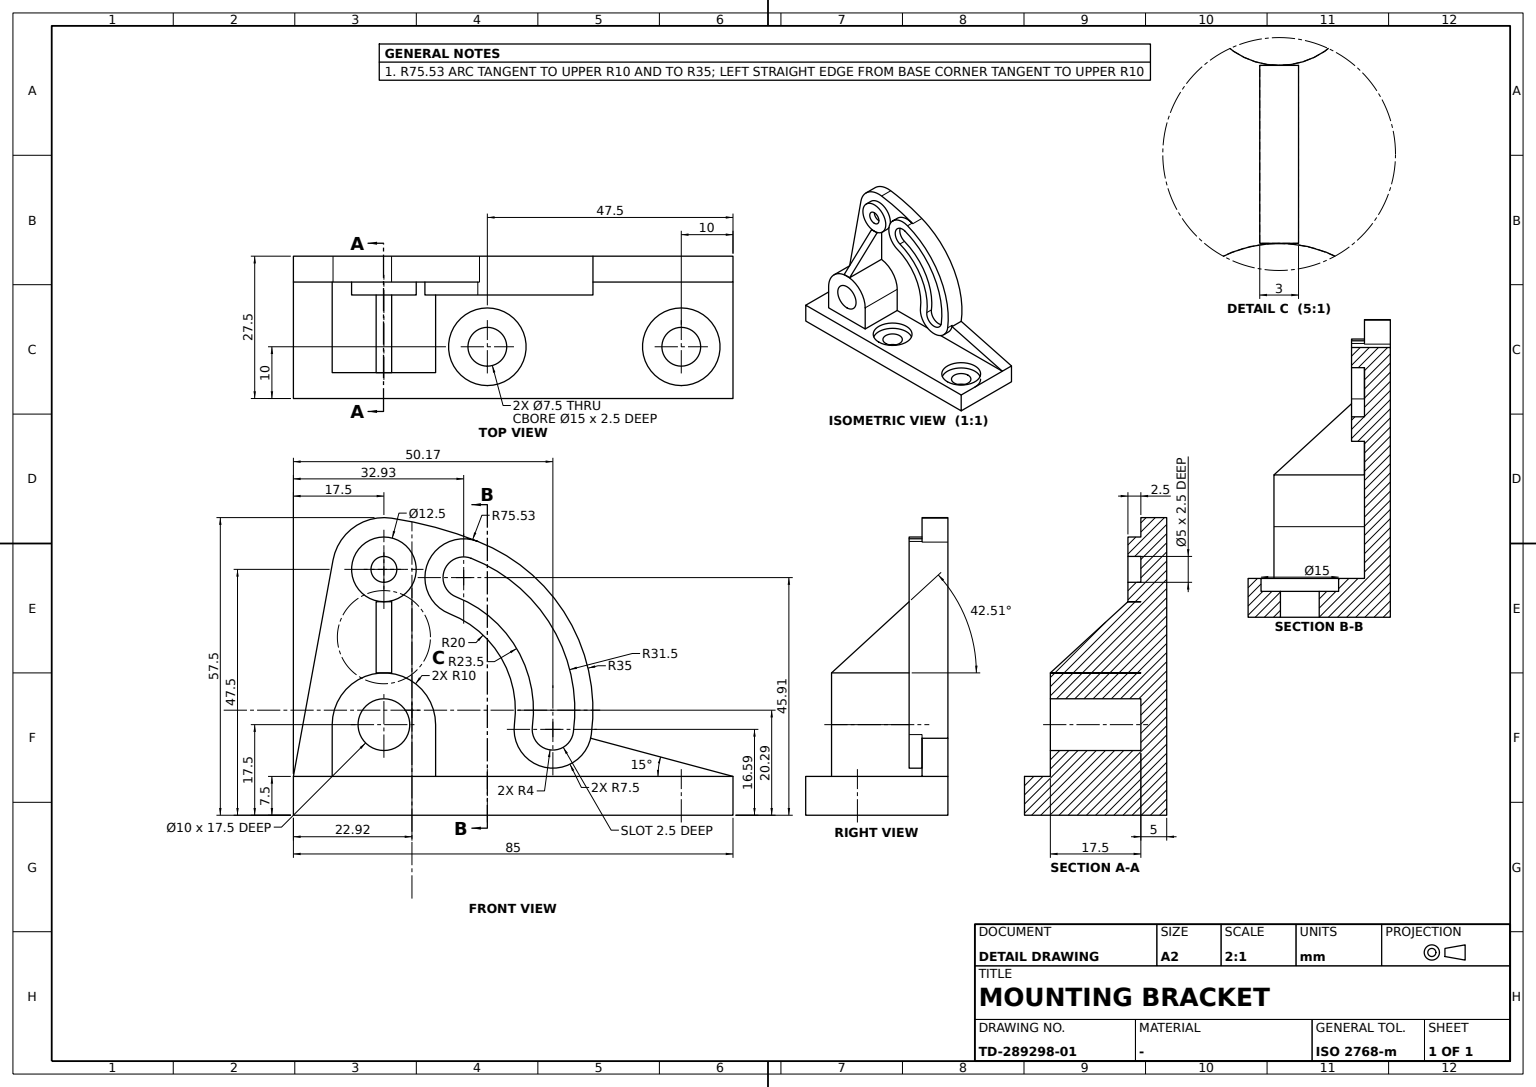
CATIA V5 part; units mm, degrees
sketch "Sketch1" plane through (0, 0, 0) normal (0, 0, 1) x (1, 0, 0)
  line L0 (13.75, 42.5) -> (13.75, -42.5)
  line L1 (13.75, -42.5) -> (-13.75, -42.5)
  line L2 (-13.75, -42.5) -> (-13.75, 42.5)
  line L3 (-13.75, 42.5) -> (13.75, 42.5)
  dimension "length L0" = 85
  dimension "length L1" = 27.5
  constraint vertical L0 y-axis
  constraint vertical L2 y-axis
  constraint horizontal L1 x-axis
  constraint horizontal L3 x-axis
  constraint equidistance L0 L2 origin
  constraint equidistance L1 L3 origin
extrude "Pad1" add sketch "Sketch1" along normal blind 7.5
sketch "Sketch2" plane through (-13.75, 0, 0) normal (-1, 0, 0) x (0, -1, 0)
  arc A0 (34.8361, 49.3033) -> (23.5195, 57.3898) centre (25, 47.5) ccw
  point P0 (25, 47.5)
  line L0 (-42.5, 7.5) -> (42.5, 7.5) construction
  line L1 (42.5, 0) -> (42.5, 7.5) construction
  line L2 (34.8361, 49.3033) -> (42.5, 7.5)
  point P1 (42.5, 7.5)
  point P2 (42.5, 7.5)
  point P3 (25, 17.5)
  line L3 (-42.5, 7.5) -> (42.5, 7.5) construction
  line L4 (42.5, 0) -> (42.5, 7.5) construction
  line L5 (-42.5, 7.5) -> (-15, 14.8686)
  point P4 (-42.5, 7.5)
  point P5 (-42.5, 7.5)
  line L6 (-42.5, 7.5) -> (42.5, 7.5) construction
  line L7 (-42.5, 7.5) -> (42.5, 7.5)
  point P6 (9.75, 46.2)
  arc A1 (-15, 14.8686) -> (6.5158, 52.7659) centre (19.5769, 20.2943) cw
  point P7 (-15, 14.8686)
  point P8 (6.5158, 52.7659)
  arc A2 (6.5158, 52.7659) -> (23.5195, 57.3898) centre (34.7021, -17.309) cw
  point P9 (6.5158, 52.7659)
  arc A3 (13.3911, 47.8559) -> (-6.4867, 9.4478) centre (25, 17.5) ccw construction
  point P10 (-15, 14.8686)
  dimension "distance P0 L0" = 40
  dimension "radius A0" = 10
  dimension "distance P0 L1" = 17.5
  dimension "distance P3 L3" = 10
  dimension "distance P3 L4" = 17.5
  dimension "angle L6 L5" = 15
  dimension "distance P6 P0 x axis" = 15.25
  dimension "radius A1" = 35
  dimension "radius A2" = 75.5312
  dimension "distance P7 P0 x axis" = 40
  constraint coincidence P2 P1
  constraint coincidence P5 P4
  constraint coincidence P7 P10
  constraint coincidence P8 P9
  constraint tangency L2 A0
  constraint tangency A0 A2
  constraint tangency A1 A2
  constraint horizontal L7 x-axis
extrude "Pad2" add sketch "Sketch2" against normal blind 5
sketch "Sketch3" plane through (-8.75, 0, 0) normal (1, 0, 0) x (0, 1, 0)
  point P0 (-6.92, 52.9252)
  point P1 (-13.2128, 47.5656)
  point P2 (6.665, 9.1574)
  point P3 (14.9168, 14.6483)
  point P4 (7.6724, 16.5895)
  point P5 (-9.5717, 45.9096)
  point P6 (-19.5769, 20.2943)
  arc A0 (-13.2128, 47.5656) -> (6.665, 9.1574) centre (-24.8217, 17.2096) cw construction
  point P7 (-19.5769, 20.2943)
  arc A1 (-11.027, 42.1837) -> (-8.1164, 49.6355) centre (-9.5717, 45.9096) cw
  arc A2 (15.104, 15.579) -> (0.2408, 17.5999) centre (7.6724, 16.5895) cw
  arc A3 (15.104, 15.579) -> (-6.843, 52.8956) centre (-19.5769, 20.2943) ccw
  arc A4 (-12.3004, 38.9236) -> (-6.843, 52.8956) centre (-9.5717, 45.9096) cw
  arc A5 (0.2408, 17.5999) -> (-12.3004, 38.9236) centre (-19.5769, 20.2943) ccw
  arc A6 (-11.027, 42.1837) -> (3.7089, 17.1283) centre (-19.5769, 20.2943) cw
  arc A7 (11.6359, 16.0506) -> (3.7089, 17.1283) centre (7.6724, 16.5895) cw
  arc A8 (-8.1164, 49.6355) -> (11.6359, 16.0506) centre (-19.5769, 20.2943) cw
  arc A9 (15, 14.8686) -> (-6.5158, 52.7659) centre (-19.5769, 20.2943) ccw construction
  dimension "radius A2" = 7.5
  dimension "radius A7" = 4
  dimension "radius A0" = 32.5
  constraint coincidence P0 A4
  constraint coincidence P1 A1
  constraint coincidence P2 A2
  constraint coincidence P3 A2
  constraint coincidence P4 A0
  constraint coincidence P5 A0
  constraint coincidence P6 P7
  constraint coincidence A3 A9
  constraint concentricity P6 A5
  constraint concentricity P6 A6
  constraint concentricity P6 A8
  constraint tangency A1 A6
  constraint tangency A1 A8
  constraint tangency A2 A3
  constraint tangency A2 A5
  constraint tangency A3 A4
  constraint tangency A4 A5
  constraint tangency A6 A7
  constraint tangency A7 A8
extrude "Pad3" add sketch "Sketch3" along normal blind 2.5
sketch "Sketch4" plane through (-8.75, 0, 0) normal (1, 0, 0) x (0, 1, 0)
  arc A0 (-15, 17.5) -> (-35, 17.5) centre (-25, 17.5) ccw
  point P0 (-25, 17.5)
  line L0 (-42.5, 0) -> (-42.5, 7.5) construction
  line L1 (-42.5, 7.5) -> (42.5, 7.5) construction
  circle A1 centre (-25, 17.5) radius 5
  line L2 (-35, 17.5) -> (-35, 7.5)
  point P1 (-35, 7.5)
  line L3 (42.5, 7.5) -> (-42.5, 7.5) construction
  line L4 (-15, 17.5) -> (-15, 7.5)
  point P2 (-15, 7.5)
  line L5 (42.5, 7.5) -> (-42.5, 7.5) construction
  line L6 (-35, 7.5) -> (-15, 7.5)
  point P3 (-35, 7.5)
  point P4 (-15, 7.5)
  circle A2 centre (-25, 47.5) radius 6.25
  circle A3 centre (-25, 47.5) radius 2.5
  point P5 (-25, 47.5)
  line L7 (-42.5, 7.5) -> (42.5, 7.5) construction
  dimension "radius A0" = 10
  dimension "distance L0 P0" = 17.5
  dimension "distance L1 P0" = 10
  dimension "radius A1" = 5
  dimension "radius A2" = 6.25
  dimension "radius A3" = 2.5
  dimension "distance L7 P5" = 40
  dimension "distance P5 P0 x axis" = 0
  constraint vertical L2 y-axis
  constraint vertical L4 y-axis
  constraint tangency L2 A0
  constraint tangency L4 A0
  constraint coincidence P1 L3
  constraint coincidence P2 L5
  constraint coincidence P3 P1
  constraint coincidence P2 P4
  constraint horizontal L6 x-axis
  constraint concentricity A2 A3
extrude "MultiPad1 domain 1" add sketch "Sketch4" along normal blind 17.5 contours A0 L2 L6 L4
extrude "MultiPad1 domain 2" add sketch "Sketch4" along normal blind 2.5 contours A2
ref_plane "Plane1" through (0, -25, 0) normal (0, -1, 0) x (-1, 0, 0)
sketch "Sketch5" plane through (0, -25, 0) normal (0, 1, 0) x (-1, 0, 0)
  line L0 (6.25, 41.25) -> (-8.75, 27.5)
  point P0 (6.25, 41.25)
  point P1 (-8.75, 27.5)
  line L1 (6.25, 41.25) -> (6.25, 53.75) construction
  line L2 (-8.75, 17.5) -> (-8.75, 27.5) construction
  point P2 (-13.75, 7.5)
  point P3 (-13.75, 7.5)
  line L3 (-8.75, 27.5) -> (8.75, 27.5)
  line L4 (6.25, 41.25) -> (8.75, 41.25)
  line L5 (8.75, 41.25) -> (8.75, 27.5)
  dimension "distance P1 P2 y axis" = 20
  dimension "distance P0 P3 y axis" = 33.75
  dimension "length L3" = 17.5
  constraint coincidence P0 L1
  constraint coincidence P1 L2
  constraint horizontal L3 x-axis
  constraint horizontal L4 x-axis
  constraint vertical L5 y-axis
extrude "Pad4" add sketch "Sketch5" along normal mid plane 3
sketch "Sketch6" plane through (3.4986, 33.4715, 7.5) normal (0, 0, 1) x (1, 0, 0)
  point P0 (0.2514, -0.9715)
  line L0 (10.2514, 9.0285) -> (-17.2486, 9.0285) construction
  line L1 (10.2514, -75.9715) -> (10.2514, 9.0285) construction
  dimension "distance L0 P0" = 10
  dimension "distance P0 L1" = 10
hole "Hole1" at (3.75, 32.5, 7.5) direction (0, 0, -1) diameter 7.5 end through all counterbore diameter 15 counterbore depth 2.5
sketch "Sketch7" plane through (3.42, 12.2534, 7.5) normal (0, 0, 1) x (1, 0, 0)
  point P0 (0.33, -17.2534)
  line L0 (10.33, -54.7534) -> (10.33, 30.2466) construction
  line L1 (10.33, 30.2466) -> (-17.17, 30.2466) construction
  dimension "distance P0 L0" = 10
  dimension "distance P0 L1" = 47.5
hole "Hole2" at (3.75, -5, 7.5) direction (0, 0, -1) diameter 7.5 end through all counterbore diameter 15 counterbore depth 2.5
